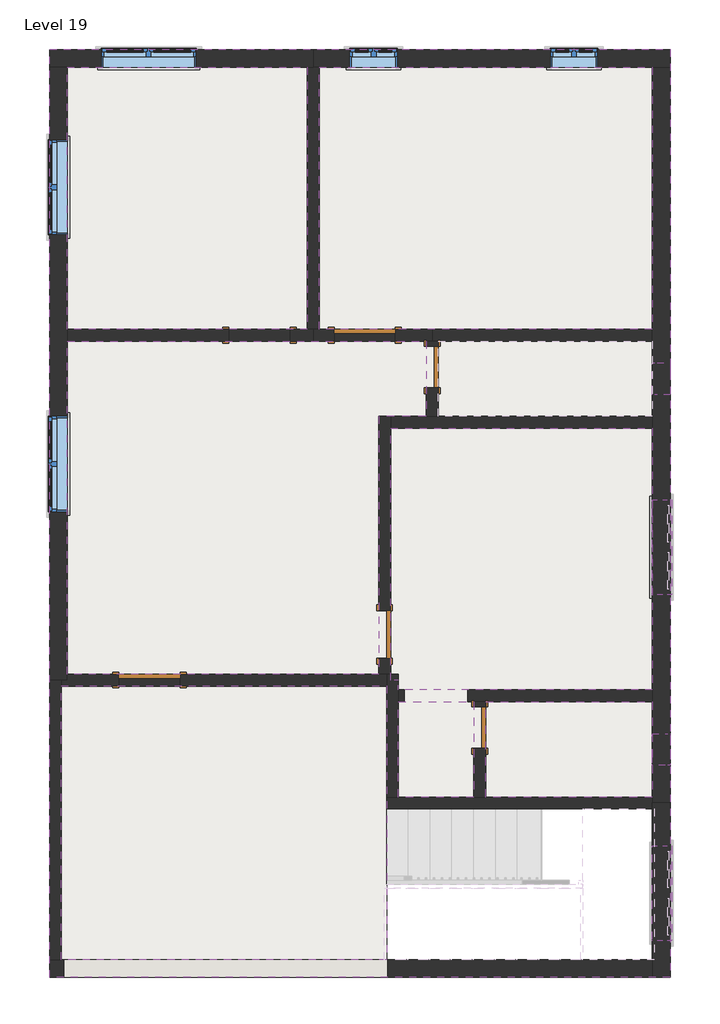
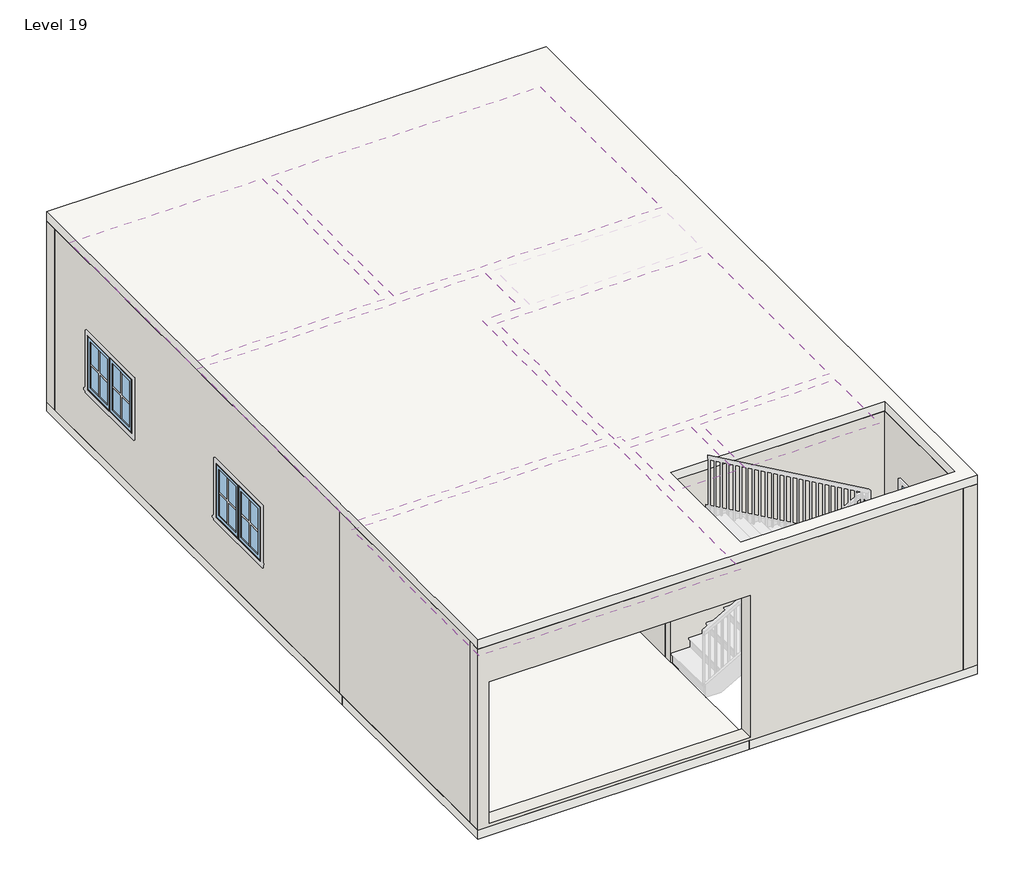
# One storey, part 1 of 2: 27 walls, 13 windows, 7 coverings, 6 doors, 3 slabs.
# Revit data of these elements (continued)
# Element 47 (IfcWindow, "Window-Casement-Double : 3'") (continued)
#   Materials on its faces: "Wood - Stained", "Glass", "Clad - White"
# Element 48 (IfcWindow, "Window-Casement-Double : 3'")
#   Mark = "77"
#   Window Inset = 0' - 0"
#   Interior Wall Closure = 0' - 2 1/4"
#   Frame Extension = 0' - 0 1/4"
#   Exterior Wall Closure = 0' - 1 1/4"
#   Interior Trim Visibility = yes
#   Exterior Trim Visibility = yes
#   Phase Created = New Construction
#   Materials on its faces: "Wood - Stained", "Glass", "Clad - White"
# Element 49 (IfcWindow, "Window-Casement-Double : 3'")
#   Mark = "78"
#   Window Inset = 0' - 0"
#   Interior Wall Closure = 0' - 2 1/4"
#   Frame Extension = 0' - 0 1/4"
#   Exterior Wall Closure = 0' - 1 1/4"
#   Interior Trim Visibility = yes
#   Exterior Trim Visibility = yes
#   Phase Created = New Construction
#   Materials on its faces: "Wood - Stained", "Glass", "Clad - White"
# Element 50 (IfcWindow, "Window-Casement-Double : 4'")
#   Mark = "66"
#   Window Inset = 0' - 0"
#   Interior Wall Closure = 0' - 2 1/4"
#   Frame Extension = 0' - 0 1/4"
#   Exterior Wall Closure = 0' - 1 1/4"
#   Interior Trim Visibility = yes
#   Exterior Trim Visibility = yes
#   Phase Created = New Construction
#   Materials on its faces: "Wood - Stained", "Glass", "Clad - White"
# Element 51 (IfcWindow, "Window-Casement-Double : 4'")
#   Mark = "67"
#   Window Inset = 0' - 0"
#   Interior Wall Closure = 0' - 2 1/4"
#   Frame Extension = 0' - 0 1/4"
#   Exterior Wall Closure = 0' - 1 1/4"
#   Interior Trim Visibility = yes
#   Exterior Trim Visibility = yes
#   Phase Created = New Construction
#   Materials on its faces: "Wood - Stained", "Glass", "Clad - White"
# Element 52 (IfcWindow, "Window-Casement-Double : 4'")
#   Mark = "68"
#   Window Inset = 0' - 0"
#   Interior Wall Closure = 0' - 2 1/4"
#   Frame Extension = 0' - 0 1/4"
#   Exterior Wall Closure = 0' - 1 1/4"
#   Interior Trim Visibility = yes
#   Exterior Trim Visibility = yes
#   Phase Created = New Construction
#   Materials on its faces: "Wood - Stained", "Glass", "Clad - White"
# Element 53 (IfcWindow, "Window-Casement-Double : 4'")
#   Mark = "69"
#   Window Inset = 0' - 0"
#   Interior Wall Closure = 0' - 2 1/4"
#   Frame Extension = 0' - 0 1/4"
#   Exterior Wall Closure = 0' - 1 1/4"
#   Interior Trim Visibility = yes
#   Exterior Trim Visibility = yes
#   Phase Created = New Construction
#   Materials on its faces: "Wood - Stained", "Glass", "Clad - White"
# Element 54 (IfcWindow, "Window-Casement-Double : 4'")
#   Mark = "70"
#   Window Inset = 0' - 0"
#   Interior Wall Closure = 0' - 2 1/4"
#   Frame Extension = 0' - 0 1/4"
#   Exterior Wall Closure = 0' - 1 1/4"
#   Interior Trim Visibility = yes
#   Exterior Trim Visibility = yes
#   Phase Created = New Construction
#   Materials on its faces: "Wood - Stained", "Glass", "Clad - White"
# Element 55 (IfcWindow, "Window-Casement-Double : 4'")
#   Mark = "75"
#   Window Inset = 0' - 0"
#   Interior Wall Closure = 0' - 2 1/4"
#   Frame Extension = 0' - 0 1/4"
#   Exterior Wall Closure = 0' - 1 1/4"
#   Interior Trim Visibility = yes
#   Exterior Trim Visibility = yes
#   Phase Created = New Construction
#   Materials on its faces: "Wood - Stained", "Glass", "Clad - White"
# Element 56 (IfcWindow, "Window-Casement-Double : 4'")
#   Mark = "76"
#   Window Inset = 0' - 0"
#   Interior Wall Closure = 0' - 2 1/4"
#   Frame Extension = 0' - 0 1/4"
#   Exterior Wall Closure = 0' - 1 1/4"
#   Interior Trim Visibility = yes
#   Exterior Trim Visibility = yes
#   Phase Created = New Construction
#   Materials on its faces: "Wood - Stained", "Glass", "Clad - White"
# Materials
#   "Default": colour RGB 127 127 127, transparency 0, Cost = 0
#   "Acoustic Ceiling Tile 24 x 48": class "Generic", colour RGB 229 229 229, transparency 0, Description = "Acoustic Ceiling Tile 24 x 48", Cost = 0
#   "Door - Panel": class "Wood", colour RGB 210 159 95, transparency 0, Cost = 0
#   "Door - Frame": colour RGB 118 70 51, transparency 0, Cost = 0
#   "Glass": class "Glass", colour RGB 0 128 192, transparency 0.75, Description = "Soda Lime Glass", Cost = 0
#   "Sash": class "Wood", colour RGB 224 178 126, transparency 0, Cost = 0
#   "Wood - Stained": class "Wood", colour RGB 224 178 126, transparency 0, Cost = 0
#   "Clad - White": class "Wood", colour RGB 242 242 238, transparency 0, Cost = 0
#   "Default Floor": colour RGB 128 128 128, transparency 0, Cost = 0
#   "TILE": class "Generic", colour RGB 120 120 120, transparency 0, Cost = 0
#   "Grass": class "Generic", colour RGB 104 137 66, transparency 0, Description = "Physical material.", Cost = 0
#   "Default Wall": colour RGB 128 128 128, transparency 0, Cost = 0
#   "WALL PAINT 4": class "Generic", colour RGB 120 120 120, transparency 0, Cost = 0
#   "MARBLE": class "Generic", colour RGB 120 120 120, transparency 0, Cost = 0
#   "WALL PAINT 5": class "Generic", colour RGB 120 120 120, transparency 0, Cost = 0
#   "WALL PAINT 2": class "Generic", colour RGB 120 120 120, transparency 0, Cost = 0
#   "WALL PAINT 3": class "Generic", colour RGB 120 120 120, transparency 0, Cost = 0
#   "WALL PAINT 1": class "Generic", colour RGB 120 120 120, transparency 0, Cost = 0
